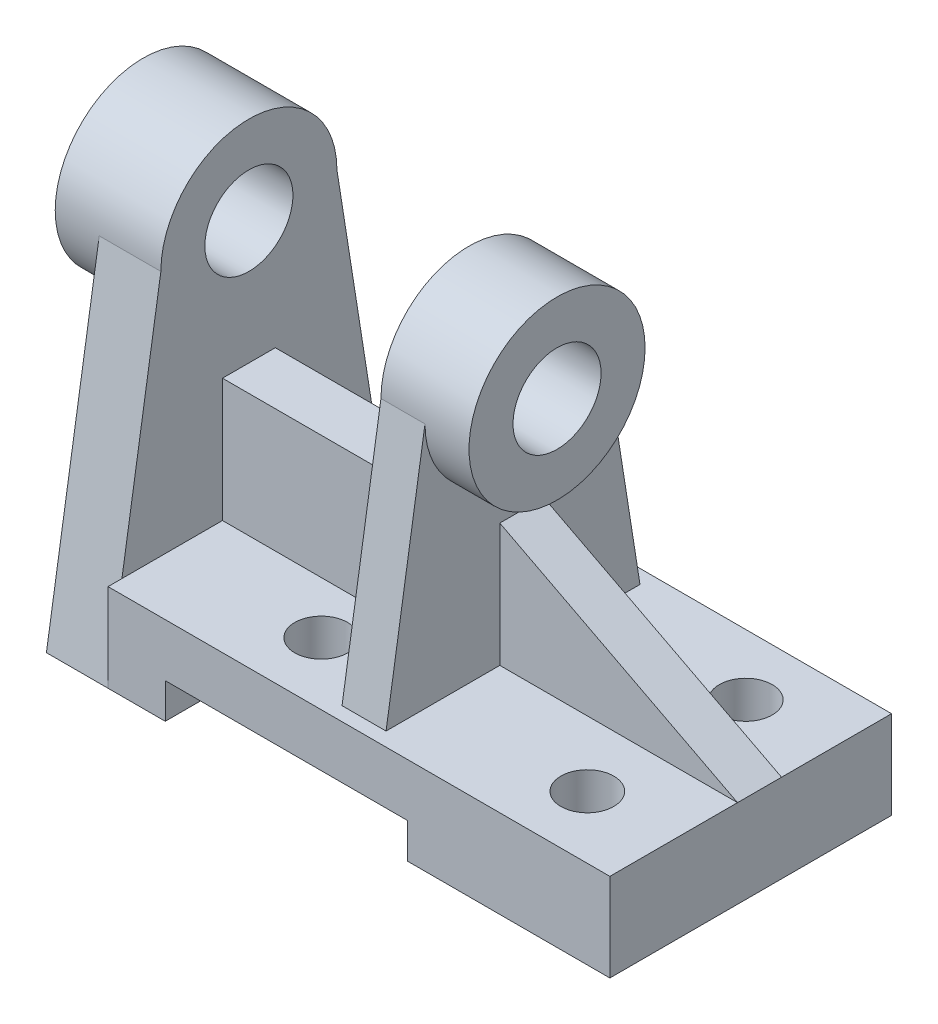
ISO-10303-21;
HEADER;
FILE_DESCRIPTION(('STEP AP214'),'2;1');
FILE_NAME('part.step','',(''),(''),'','','');
FILE_SCHEMA(('AUTOMOTIVE_DESIGN { 1 0 10303 214 1 1 1 1 }'));
ENDSEC;
DATA;
#1=APPLICATION_CONTEXT('core data for automotive mechanical design processes');
#2=APPLICATION_PROTOCOL_DEFINITION('international standard','automotive_design',2000,#1);
#3=PRODUCT_CONTEXT('',#1,'mechanical');
#4=PRODUCT('Part','Part','',(#3));
#5=PRODUCT_RELATED_PRODUCT_CATEGORY('part','',(#4));
#6=PRODUCT_DEFINITION_FORMATION('','',#4);
#7=PRODUCT_DEFINITION_CONTEXT('part definition',#1,'design');
#8=PRODUCT_DEFINITION('design','',#6,#7);
#9=PRODUCT_DEFINITION_SHAPE('','',#8);
#10=(LENGTH_UNIT() NAMED_UNIT(*) SI_UNIT(.MILLI.,.METRE.));
#11=(NAMED_UNIT(*) PLANE_ANGLE_UNIT() SI_UNIT($,.RADIAN.));
#12=(NAMED_UNIT(*) SI_UNIT($,.STERADIAN.) SOLID_ANGLE_UNIT());
#13=UNCERTAINTY_MEASURE_WITH_UNIT(LENGTH_MEASURE(1.E-05),#10,'distance_accuracy_value','');
#14=(GEOMETRIC_REPRESENTATION_CONTEXT(3) GLOBAL_UNCERTAINTY_ASSIGNED_CONTEXT((#13)) GLOBAL_UNIT_ASSIGNED_CONTEXT((#10,
#11,#12)) REPRESENTATION_CONTEXT('',''));
#15=CARTESIAN_POINT('',(0.,0.,0.));
#16=DIRECTION('',(0.,0.,1.));
#17=DIRECTION('',(1.,0.,0.));
#18=AXIS2_PLACEMENT_3D('',#15,#16,#17);
#19=CARTESIAN_POINT('',(-64.,10.,64.));
#20=DIRECTION('',(0.,-1.,0.));
#21=DIRECTION('',(1.,0.,0.));
#22=AXIS2_PLACEMENT_3D('',#19,#20,#21);
#23=PLANE('',#22);
#24=CARTESIAN_POINT('',(-15.7437869593848,10.,49.8283194926064));
#25=DIRECTION('',(0.,1.,0.));
#26=DIRECTION('',(-1.,0.,0.));
#27=AXIS2_PLACEMENT_3D('',#24,#25,#26);
#28=CIRCLE('',#27,6.);
#29=CARTESIAN_POINT('',(-21.7437869593848,10.,49.8283194926064));
#30=VERTEX_POINT('',#29);
#31=EDGE_CURVE('E223',#30,#30,#28,.T.);
#32=ORIENTED_EDGE('',*,*,#31,.F.);
#33=EDGE_LOOP('',(#32));
#34=FACE_BOUND('',#33,.T.);
#35=CARTESIAN_POINT('',(44.7041403429973,10.,49.8283194926064));
#36=DIRECTION('',(0.,1.,0.));
#37=DIRECTION('',(-1.,0.,0.));
#38=AXIS2_PLACEMENT_3D('',#35,#36,#37);
#39=CIRCLE('',#38,6.);
#40=CARTESIAN_POINT('',(38.7041403429973,10.,49.8283194926064));
#41=VERTEX_POINT('',#40);
#42=EDGE_CURVE('E495',#41,#41,#39,.T.);
#43=ORIENTED_EDGE('',*,*,#42,.F.);
#44=EDGE_LOOP('',(#43));
#45=FACE_BOUND('',#44,.T.);
#46=DIRECTION('',(0.,0.,-1.));
#47=VECTOR('',#46,1.);
#48=CARTESIAN_POINT('',(64.,10.,64.));
#49=LINE('',#48,#47);
#50=CARTESIAN_POINT('',(64.,10.,64.));
#51=VERTEX_POINT('',#50);
#52=CARTESIAN_POINT('',(64.,10.,35.));
#53=VERTEX_POINT('',#52);
#54=EDGE_CURVE('E385',#51,#53,#49,.T.);
#55=ORIENTED_EDGE('',*,*,#54,.T.);
#56=DIRECTION('',(-1.,0.,0.));
#57=VECTOR('',#56,1.);
#58=CARTESIAN_POINT('',(-64.,10.,35.));
#59=LINE('',#58,#57);
#60=CARTESIAN_POINT('',(10.,10.,35.));
#61=VERTEX_POINT('',#60);
#62=EDGE_CURVE('E236',#53,#61,#59,.T.);
#63=ORIENTED_EDGE('',*,*,#62,.T.);
#64=DIRECTION('',(0.,0.,-1.));
#65=VECTOR('',#64,1.);
#66=CARTESIAN_POINT('',(10.,10.,60.8421052631579));
#67=LINE('',#66,#65);
#68=CARTESIAN_POINT('',(10.,10.,60.8421052631579));
#69=VERTEX_POINT('',#68);
#70=EDGE_CURVE('E256',#69,#61,#67,.T.);
#71=ORIENTED_EDGE('',*,*,#70,.F.);
#72=DIRECTION('',(-1.,0.,0.));
#73=VECTOR('',#72,1.);
#74=CARTESIAN_POINT('',(10.,10.,60.8421052631579));
#75=LINE('',#74,#73);
#76=CARTESIAN_POINT('',(0.,10.,60.8421052631579));
#77=VERTEX_POINT('',#76);
#78=EDGE_CURVE('E271',#69,#77,#75,.T.);
#79=ORIENTED_EDGE('',*,*,#78,.T.);
#80=DIRECTION('',(0.,0.,-1.));
#81=VECTOR('',#80,1.);
#82=CARTESIAN_POINT('',(0.,10.,60.8421052631579));
#83=LINE('',#82,#81);
#84=CARTESIAN_POINT('',(0.,10.,38.));
#85=VERTEX_POINT('',#84);
#86=EDGE_CURVE('E264',#77,#85,#83,.T.);
#87=ORIENTED_EDGE('',*,*,#86,.T.);
#88=DIRECTION('',(1.,0.,0.));
#89=VECTOR('',#88,1.);
#90=CARTESIAN_POINT('',(0.,10.,38.));
#91=LINE('',#90,#89);
#92=CARTESIAN_POINT('',(-50.,10.,38.));
#93=VERTEX_POINT('',#92);
#94=EDGE_CURVE('E278',#93,#85,#91,.T.);
#95=ORIENTED_EDGE('',*,*,#94,.F.);
#96=DIRECTION('',(0.,0.,-1.));
#97=VECTOR('',#96,1.);
#98=CARTESIAN_POINT('',(-50.,10.,0.));
#99=LINE('',#98,#97);
#100=CARTESIAN_POINT('',(-50.,10.,60.8421052631579));
#101=VERTEX_POINT('',#100);
#102=EDGE_CURVE('E344',#101,#93,#99,.T.);
#103=ORIENTED_EDGE('',*,*,#102,.F.);
#104=CARTESIAN_POINT('',(-50.,10.,64.));
#105=VERTEX_POINT('',#104);
#106=EDGE_CURVE('E336',#105,#101,#99,.T.);
#107=ORIENTED_EDGE('',*,*,#106,.F.);
#108=DIRECTION('',(-1.,0.,0.));
#109=VECTOR('',#108,1.);
#110=CARTESIAN_POINT('',(-64.,10.,64.));
#111=LINE('',#110,#109);
#112=EDGE_CURVE('E359',#51,#105,#111,.T.);
#113=ORIENTED_EDGE('',*,*,#112,.F.);
#114=EDGE_LOOP('',(#55,#63,#71,#79,#87,#95,#103,#107,#113));
#115=FACE_BOUND('',#114,.T.);
#116=ADVANCED_FACE('F39',(#34,#45,#115),#23,.F.);
#117=CARTESIAN_POINT('',(0.,0.,0.));
#118=DIRECTION('',(1.,0.,0.));
#119=DIRECTION('',(0.,0.,-1.));
#120=AXIS2_PLACEMENT_3D('',#117,#118,#119);
#121=PLANE('',#120);
#122=DIRECTION('',(0.,-1.,0.));
#123=VECTOR('',#122,1.);
#124=CARTESIAN_POINT('',(0.,38.,26.));
#125=LINE('',#124,#123);
#126=CARTESIAN_POINT('',(0.,38.,26.));
#127=VERTEX_POINT('',#126);
#128=CARTESIAN_POINT('',(0.,10.,26.));
#129=VERTEX_POINT('',#128);
#130=EDGE_CURVE('E294',#127,#129,#125,.T.);
#131=ORIENTED_EDGE('',*,*,#130,.F.);
#132=DIRECTION('',(0.,0.,-1.));
#133=VECTOR('',#132,1.);
#134=CARTESIAN_POINT('',(0.,38.,26.));
#135=LINE('',#134,#133);
#136=CARTESIAN_POINT('',(0.,38.,38.));
#137=VERTEX_POINT('',#136);
#138=EDGE_CURVE('E284',#137,#127,#135,.T.);
#139=ORIENTED_EDGE('',*,*,#138,.F.);
#140=DIRECTION('',(0.,-1.,0.));
#141=VECTOR('',#140,1.);
#142=CARTESIAN_POINT('',(0.,38.,38.));
#143=LINE('',#142,#141);
#144=EDGE_CURVE('E296',#137,#85,#143,.T.);
#145=ORIENTED_EDGE('',*,*,#144,.T.);
#146=ORIENTED_EDGE('',*,*,#86,.F.);
#147=DIRECTION('',(0.,-0.987762965329069,0.155962573473011));
#148=VECTOR('',#147,1.);
#149=CARTESIAN_POINT('',(0.,66.,52.));
#150=LINE('',#149,#148);
#151=CARTESIAN_POINT('',(0.,66.,52.));
#152=VERTEX_POINT('',#151);
#153=EDGE_CURVE('E249',#152,#77,#150,.T.);
#154=ORIENTED_EDGE('',*,*,#153,.F.);
#155=CARTESIAN_POINT('',(0.,66.,32.));
#156=DIRECTION('',(1.,0.,0.));
#157=DIRECTION('',(0.,0.,-1.));
#158=AXIS2_PLACEMENT_3D('',#155,#156,#157);
#159=CIRCLE('',#158,20.);
#160=CARTESIAN_POINT('',(0.,66.,12.));
#161=VERTEX_POINT('',#160);
#162=EDGE_CURVE('E242',#161,#152,#159,.T.);
#163=ORIENTED_EDGE('',*,*,#162,.F.);
#164=DIRECTION('',(0.,0.987762965329069,0.155962573473011));
#165=VECTOR('',#164,1.);
#166=CARTESIAN_POINT('',(0.,10.,3.15789473684211));
#167=LINE('',#166,#165);
#168=CARTESIAN_POINT('',(0.,10.,3.15789473684211));
#169=VERTEX_POINT('',#168);
#170=EDGE_CURVE('E259',#169,#161,#167,.T.);
#171=ORIENTED_EDGE('',*,*,#170,.F.);
#172=EDGE_CURVE('E261',#129,#169,#83,.T.);
#173=ORIENTED_EDGE('',*,*,#172,.F.);
#174=EDGE_LOOP('',(#131,#139,#145,#146,#154,#163,#171,#173));
#175=FACE_BOUND('',#174,.T.);
#176=CARTESIAN_POINT('',(0.,66.,32.));
#177=DIRECTION('',(1.,0.,0.));
#178=DIRECTION('',(0.,0.,-1.));
#179=AXIS2_PLACEMENT_3D('',#176,#177,#178);
#180=CIRCLE('',#179,10.);
#181=CARTESIAN_POINT('',(0.,66.,22.));
#182=VERTEX_POINT('',#181);
#183=EDGE_CURVE('E239',#182,#182,#180,.T.);
#184=ORIENTED_EDGE('',*,*,#183,.T.);
#185=EDGE_LOOP('',(#184));
#186=FACE_BOUND('',#185,.T.);
#187=ADVANCED_FACE('F411',(#175,#186),#121,.F.);
#188=CARTESIAN_POINT('',(44.7041403429973,10.,13.8283194926064));
#189=DIRECTION('',(0.,1.,0.));
#190=DIRECTION('',(-1.,0.,0.));
#191=AXIS2_PLACEMENT_3D('',#188,#189,#190);
#192=CIRCLE('',#191,6.);
#193=CARTESIAN_POINT('',(38.7041403429973,10.,13.8283194926064));
#194=VERTEX_POINT('',#193);
#195=EDGE_CURVE('E235',#194,#194,#192,.T.);
#196=ORIENTED_EDGE('',*,*,#195,.F.);
#197=EDGE_LOOP('',(#196));
#198=FACE_BOUND('',#197,.T.);
#199=CARTESIAN_POINT('',(-15.7437869593848,10.,13.8283194926064));
#200=DIRECTION('',(0.,1.,0.));
#201=DIRECTION('',(-1.,0.,0.));
#202=AXIS2_PLACEMENT_3D('',#199,#200,#201);
#203=CIRCLE('',#202,6.);
#204=CARTESIAN_POINT('',(-21.7437869593848,10.,13.8283194926064));
#205=VERTEX_POINT('',#204);
#206=EDGE_CURVE('E216',#205,#205,#203,.T.);
#207=ORIENTED_EDGE('',*,*,#206,.F.);
#208=EDGE_LOOP('',(#207));
#209=FACE_BOUND('',#208,.T.);
#210=ORIENTED_EDGE('',*,*,#172,.T.);
#211=DIRECTION('',(-1.,0.,0.));
#212=VECTOR('',#211,1.);
#213=CARTESIAN_POINT('',(10.,10.,3.15789473684211));
#214=LINE('',#213,#212);
#215=CARTESIAN_POINT('',(10.,10.,3.15789473684211));
#216=VERTEX_POINT('',#215);
#217=EDGE_CURVE('E269',#216,#169,#214,.T.);
#218=ORIENTED_EDGE('',*,*,#217,.F.);
#219=CARTESIAN_POINT('',(10.,10.,25.));
#220=VERTEX_POINT('',#219);
#221=EDGE_CURVE('E253',#220,#216,#67,.T.);
#222=ORIENTED_EDGE('',*,*,#221,.F.);
#223=DIRECTION('',(-1.,0.,0.));
#224=VECTOR('',#223,1.);
#225=CARTESIAN_POINT('',(-64.,10.,25.));
#226=LINE('',#225,#224);
#227=CARTESIAN_POINT('',(64.,10.,25.));
#228=VERTEX_POINT('',#227);
#229=EDGE_CURVE('E57',#228,#220,#226,.T.);
#230=ORIENTED_EDGE('',*,*,#229,.F.);
#231=CARTESIAN_POINT('',(64.,10.,0.));
#232=VERTEX_POINT('',#231);
#233=EDGE_CURVE('E382',#228,#232,#49,.T.);
#234=ORIENTED_EDGE('',*,*,#233,.T.);
#235=DIRECTION('',(-1.,0.,0.));
#236=VECTOR('',#235,1.);
#237=CARTESIAN_POINT('',(-64.,10.,0.));
#238=LINE('',#237,#236);
#239=CARTESIAN_POINT('',(-50.,10.,0.));
#240=VERTEX_POINT('',#239);
#241=EDGE_CURVE('E371',#232,#240,#238,.T.);
#242=ORIENTED_EDGE('',*,*,#241,.T.);
#243=DIRECTION('',(0.,0.,-1.));
#244=VECTOR('',#243,1.);
#245=CARTESIAN_POINT('',(-50.,10.,64.));
#246=LINE('',#245,#244);
#247=CARTESIAN_POINT('',(-50.,10.,3.15789473684211));
#248=VERTEX_POINT('',#247);
#249=EDGE_CURVE('E309',#248,#240,#246,.T.);
#250=ORIENTED_EDGE('',*,*,#249,.F.);
#251=CARTESIAN_POINT('',(-50.,10.,26.));
#252=VERTEX_POINT('',#251);
#253=EDGE_CURVE('E340',#252,#248,#99,.T.);
#254=ORIENTED_EDGE('',*,*,#253,.F.);
#255=DIRECTION('',(-1.,0.,0.));
#256=VECTOR('',#255,1.);
#257=CARTESIAN_POINT('',(-50.,10.,26.));
#258=LINE('',#257,#256);
#259=EDGE_CURVE('E285',#129,#252,#258,.T.);
#260=ORIENTED_EDGE('',*,*,#259,.F.);
#261=EDGE_LOOP('',(#210,#218,#222,#230,#234,#242,#250,#254,#260));
#262=FACE_BOUND('',#261,.T.);
#263=ADVANCED_FACE('F430',(#198,#209,#262),#23,.F.);
#264=CARTESIAN_POINT('',(-50.,66.,0.));
#265=DIRECTION('',(-1.,0.,0.));
#266=DIRECTION('',(0.,-1.,0.));
#267=AXIS2_PLACEMENT_3D('',#264,#265,#266);
#268=PLANE('',#267);
#269=CARTESIAN_POINT('',(-50.,66.,32.));
#270=DIRECTION('',(-1.,0.,0.));
#271=DIRECTION('',(0.,0.,1.));
#272=AXIS2_PLACEMENT_3D('',#269,#270,#271);
#273=CIRCLE('',#272,10.);
#274=CARTESIAN_POINT('',(-50.,66.,42.));
#275=VERTEX_POINT('',#274);
#276=EDGE_CURVE('E325',#275,#275,#273,.T.);
#277=ORIENTED_EDGE('',*,*,#276,.T.);
#278=EDGE_LOOP('',(#277));
#279=FACE_BOUND('',#278,.T.);
#280=DIRECTION('',(0.,-1.,0.));
#281=VECTOR('',#280,1.);
#282=CARTESIAN_POINT('',(-50.,38.,38.));
#283=LINE('',#282,#281);
#284=CARTESIAN_POINT('',(-50.,38.,38.));
#285=VERTEX_POINT('',#284);
#286=EDGE_CURVE('E297',#285,#93,#283,.T.);
#287=ORIENTED_EDGE('',*,*,#286,.F.);
#288=DIRECTION('',(0.,0.,1.));
#289=VECTOR('',#288,1.);
#290=CARTESIAN_POINT('',(-50.,38.,38.));
#291=LINE('',#290,#289);
#292=CARTESIAN_POINT('',(-50.,38.,26.));
#293=VERTEX_POINT('',#292);
#294=EDGE_CURVE('E63',#293,#285,#291,.T.);
#295=ORIENTED_EDGE('',*,*,#294,.F.);
#296=DIRECTION('',(0.,-1.,0.));
#297=VECTOR('',#296,1.);
#298=CARTESIAN_POINT('',(-50.,38.,26.));
#299=LINE('',#298,#297);
#300=EDGE_CURVE('E288',#293,#252,#299,.T.);
#301=ORIENTED_EDGE('',*,*,#300,.T.);
#302=ORIENTED_EDGE('',*,*,#253,.T.);
#303=DIRECTION('',(0.,-0.987762965329069,-0.155962573473011));
#304=VECTOR('',#303,1.);
#305=CARTESIAN_POINT('',(-50.,-0.243243243243243,1.54054054054054));
#306=LINE('',#305,#304);
#307=CARTESIAN_POINT('',(-50.,66.,12.));
#308=VERTEX_POINT('',#307);
#309=EDGE_CURVE('E302',#308,#248,#306,.T.);
#310=ORIENTED_EDGE('',*,*,#309,.F.);
#311=CARTESIAN_POINT('',(-50.,66.,32.));
#312=DIRECTION('',(-1.,0.,0.));
#313=DIRECTION('',(0.,0.,1.));
#314=AXIS2_PLACEMENT_3D('',#311,#312,#313);
#315=CIRCLE('',#314,20.);
#316=CARTESIAN_POINT('',(-50.,66.,52.));
#317=VERTEX_POINT('',#316);
#318=EDGE_CURVE('E328',#317,#308,#315,.T.);
#319=ORIENTED_EDGE('',*,*,#318,.F.);
#320=DIRECTION('',(0.,0.987762965329069,-0.155962573473011));
#321=VECTOR('',#320,1.);
#322=CARTESIAN_POINT('',(-50.,9.61621621621621,60.9027027027027));
#323=LINE('',#322,#321);
#324=EDGE_CURVE('E319',#101,#317,#323,.T.);
#325=ORIENTED_EDGE('',*,*,#324,.F.);
#326=ORIENTED_EDGE('',*,*,#102,.T.);
#327=EDGE_LOOP('',(#287,#295,#301,#302,#310,#319,#325,#326));
#328=FACE_BOUND('',#327,.T.);
#329=ADVANCED_FACE('F446',(#279,#328),#268,.F.);
#330=CARTESIAN_POINT('',(0.,0.,64.));
#331=DIRECTION('',(0.,0.,1.));
#332=DIRECTION('',(1.,0.,0.));
#333=AXIS2_PLACEMENT_3D('',#330,#331,#332);
#334=PLANE('',#333);
#335=ORIENTED_EDGE('',*,*,#112,.T.);
#336=DIRECTION('',(0.,1.,0.));
#337=VECTOR('',#336,1.);
#338=CARTESIAN_POINT('',(-50.,0.,64.));
#339=LINE('',#338,#337);
#340=CARTESIAN_POINT('',(-50.,-9.99999999999999,64.));
#341=VERTEX_POINT('',#340);
#342=EDGE_CURVE('E313',#341,#105,#339,.T.);
#343=ORIENTED_EDGE('',*,*,#342,.F.);
#344=DIRECTION('',(1.,0.,0.));
#345=VECTOR('',#344,1.);
#346=CARTESIAN_POINT('',(-64.,-9.99999999999999,64.));
#347=LINE('',#346,#345);
#348=CARTESIAN_POINT('',(-37.,-9.99999999999999,64.));
#349=VERTEX_POINT('',#348);
#350=EDGE_CURVE('E368',#341,#349,#347,.T.);
#351=ORIENTED_EDGE('',*,*,#350,.T.);
#352=DIRECTION('',(0.,-1.,0.));
#353=VECTOR('',#352,1.);
#354=CARTESIAN_POINT('',(-37.,-9.99999999999999,64.));
#355=LINE('',#354,#353);
#356=CARTESIAN_POINT('',(-37.,-1.99999999999999,64.));
#357=VERTEX_POINT('',#356);
#358=EDGE_CURVE('E342',#357,#349,#355,.T.);
#359=ORIENTED_EDGE('',*,*,#358,.F.);
#360=DIRECTION('',(-1.,0.,0.));
#361=VECTOR('',#360,1.);
#362=CARTESIAN_POINT('',(-37.,-1.99999999999999,64.));
#363=LINE('',#362,#361);
#364=CARTESIAN_POINT('',(18.,-1.99999999999999,64.));
#365=VERTEX_POINT('',#364);
#366=EDGE_CURVE('E345',#365,#357,#363,.T.);
#367=ORIENTED_EDGE('',*,*,#366,.F.);
#368=DIRECTION('',(0.,1.,0.));
#369=VECTOR('',#368,1.);
#370=CARTESIAN_POINT('',(18.,-1.99999999999999,64.));
#371=LINE('',#370,#369);
#372=CARTESIAN_POINT('',(18.,-9.99999999999999,64.));
#373=VERTEX_POINT('',#372);
#374=EDGE_CURVE('E338',#373,#365,#371,.T.);
#375=ORIENTED_EDGE('',*,*,#374,.F.);
#376=CARTESIAN_POINT('',(64.,-9.99999999999999,64.));
#377=VERTEX_POINT('',#376);
#378=EDGE_CURVE('E364',#373,#377,#347,.T.);
#379=ORIENTED_EDGE('',*,*,#378,.T.);
#380=DIRECTION('',(0.,1.,0.));
#381=VECTOR('',#380,1.);
#382=CARTESIAN_POINT('',(64.,10.,64.));
#383=LINE('',#382,#381);
#384=EDGE_CURVE('E357',#377,#51,#383,.T.);
#385=ORIENTED_EDGE('',*,*,#384,.T.);
#386=EDGE_LOOP('',(#335,#343,#351,#359,#367,#375,#379,#385));
#387=FACE_BOUND('',#386,.T.);
#388=ADVANCED_FACE('F485',(#387),#334,.T.);
#389=CARTESIAN_POINT('',(0.,0.,0.));
#390=DIRECTION('',(0.,0.,1.));
#391=DIRECTION('',(1.,0.,0.));
#392=AXIS2_PLACEMENT_3D('',#389,#390,#391);
#393=PLANE('',#392);
#394=DIRECTION('',(0.,-1.,0.));
#395=VECTOR('',#394,1.);
#396=CARTESIAN_POINT('',(-50.,0.,0.));
#397=LINE('',#396,#395);
#398=CARTESIAN_POINT('',(-50.,-9.99999999999999,0.));
#399=VERTEX_POINT('',#398);
#400=EDGE_CURVE('E310',#240,#399,#397,.T.);
#401=ORIENTED_EDGE('',*,*,#400,.F.);
#402=ORIENTED_EDGE('',*,*,#241,.F.);
#403=DIRECTION('',(0.,1.,0.));
#404=VECTOR('',#403,1.);
#405=CARTESIAN_POINT('',(64.,10.,0.));
#406=LINE('',#405,#404);
#407=CARTESIAN_POINT('',(64.,-9.99999999999999,0.));
#408=VERTEX_POINT('',#407);
#409=EDGE_CURVE('E358',#408,#232,#406,.T.);
#410=ORIENTED_EDGE('',*,*,#409,.F.);
#411=DIRECTION('',(1.,0.,0.));
#412=VECTOR('',#411,1.);
#413=CARTESIAN_POINT('',(-64.,-9.99999999999999,0.));
#414=LINE('',#413,#412);
#415=CARTESIAN_POINT('',(18.,-9.99999999999999,0.));
#416=VERTEX_POINT('',#415);
#417=EDGE_CURVE('E372',#416,#408,#414,.T.);
#418=ORIENTED_EDGE('',*,*,#417,.F.);
#419=DIRECTION('',(0.,-1.,0.));
#420=VECTOR('',#419,1.);
#421=CARTESIAN_POINT('',(18.,0.,0.));
#422=LINE('',#421,#420);
#423=CARTESIAN_POINT('',(18.,-1.99999999999999,0.));
#424=VERTEX_POINT('',#423);
#425=EDGE_CURVE('E393',#424,#416,#422,.T.);
#426=ORIENTED_EDGE('',*,*,#425,.F.);
#427=DIRECTION('',(1.,0.,0.));
#428=VECTOR('',#427,1.);
#429=CARTESIAN_POINT('',(0.,-1.99999999999999,0.));
#430=LINE('',#429,#428);
#431=CARTESIAN_POINT('',(-37.,-1.99999999999999,0.));
#432=VERTEX_POINT('',#431);
#433=EDGE_CURVE('E390',#432,#424,#430,.T.);
#434=ORIENTED_EDGE('',*,*,#433,.F.);
#435=DIRECTION('',(0.,1.,0.));
#436=VECTOR('',#435,1.);
#437=CARTESIAN_POINT('',(-37.,0.,0.));
#438=LINE('',#437,#436);
#439=CARTESIAN_POINT('',(-37.,-9.99999999999999,0.));
#440=VERTEX_POINT('',#439);
#441=EDGE_CURVE('E383',#440,#432,#438,.T.);
#442=ORIENTED_EDGE('',*,*,#441,.F.);
#443=EDGE_CURVE('E380',#399,#440,#414,.T.);
#444=ORIENTED_EDGE('',*,*,#443,.F.);
#445=EDGE_LOOP('',(#401,#402,#410,#418,#426,#434,#442,#444));
#446=FACE_BOUND('',#445,.T.);
#447=ADVANCED_FACE('F431',(#446),#393,.F.);
#448=CARTESIAN_POINT('',(-64.,10.,64.));
#449=DIRECTION('',(1.,0.,0.));
#450=DIRECTION('',(0.,0.,-1.));
#451=AXIS2_PLACEMENT_3D('',#448,#449,#450);
#452=PLANE('',#451);
#453=DIRECTION('',(0.,0.987762965329069,-0.155962573473011));
#454=VECTOR('',#453,1.);
#455=CARTESIAN_POINT('',(-64.,9.61621621621621,60.9027027027027));
#456=LINE('',#455,#454);
#457=CARTESIAN_POINT('',(-64.,-9.99999999999999,64.));
#458=VERTEX_POINT('',#457);
#459=CARTESIAN_POINT('',(-64.,66.,52.));
#460=VERTEX_POINT('',#459);
#461=EDGE_CURVE('E303',#458,#460,#456,.T.);
#462=ORIENTED_EDGE('',*,*,#461,.T.);
#463=CARTESIAN_POINT('',(-64.,66.,32.));
#464=DIRECTION('',(1.,0.,0.));
#465=DIRECTION('',(0.,0.,-1.));
#466=AXIS2_PLACEMENT_3D('',#463,#464,#465);
#467=CIRCLE('',#466,20.);
#468=CARTESIAN_POINT('',(-64.,66.,12.));
#469=VERTEX_POINT('',#468);
#470=EDGE_CURVE('E334',#469,#460,#467,.F.);
#471=ORIENTED_EDGE('',*,*,#470,.F.);
#472=DIRECTION('',(0.,-0.987762965329069,-0.155962573473011));
#473=VECTOR('',#472,1.);
#474=CARTESIAN_POINT('',(-64.,-0.243243243243243,1.54054054054054));
#475=LINE('',#474,#473);
#476=CARTESIAN_POINT('',(-64.,-9.99999999999999,0.));
#477=VERTEX_POINT('',#476);
#478=EDGE_CURVE('E311',#469,#477,#475,.T.);
#479=ORIENTED_EDGE('',*,*,#478,.T.);
#480=DIRECTION('',(0.,0.,-1.));
#481=VECTOR('',#480,1.);
#482=CARTESIAN_POINT('',(-64.,-9.99999999999999,64.));
#483=LINE('',#482,#481);
#484=EDGE_CURVE('E378',#458,#477,#483,.T.);
#485=ORIENTED_EDGE('',*,*,#484,.F.);
#486=EDGE_LOOP('',(#462,#471,#479,#485));
#487=FACE_BOUND('',#486,.T.);
#488=ADVANCED_FACE('F566',(#487),#452,.F.);
#489=CARTESIAN_POINT('',(-64.,-9.99999999999999,64.));
#490=DIRECTION('',(0.,1.,0.));
#491=DIRECTION('',(0.,0.,1.));
#492=AXIS2_PLACEMENT_3D('',#489,#490,#491);
#493=PLANE('',#492);
#494=CARTESIAN_POINT('',(44.7041403429973,-9.99999999999999,13.8283194926064));
#495=DIRECTION('',(0.,1.,0.));
#496=DIRECTION('',(-1.,0.,0.));
#497=AXIS2_PLACEMENT_3D('',#494,#495,#496);
#498=CIRCLE('',#497,6.);
#499=CARTESIAN_POINT('',(38.7041403429973,-9.99999999999999,13.8283194926064));
#500=VERTEX_POINT('',#499);
#501=EDGE_CURVE('E226',#500,#500,#498,.T.);
#502=ORIENTED_EDGE('',*,*,#501,.T.);
#503=EDGE_LOOP('',(#502));
#504=FACE_BOUND('',#503,.T.);
#505=CARTESIAN_POINT('',(44.7041403429973,-9.99999999999999,49.8283194926064));
#506=DIRECTION('',(0.,1.,0.));
#507=DIRECTION('',(-1.,0.,0.));
#508=AXIS2_PLACEMENT_3D('',#505,#506,#507);
#509=CIRCLE('',#508,6.);
#510=CARTESIAN_POINT('',(38.7041403429973,-9.99999999999999,49.8283194926064));
#511=VERTEX_POINT('',#510);
#512=EDGE_CURVE('E490',#511,#511,#509,.T.);
#513=ORIENTED_EDGE('',*,*,#512,.T.);
#514=EDGE_LOOP('',(#513));
#515=FACE_BOUND('',#514,.T.);
#516=DIRECTION('',(0.,0.,-1.));
#517=VECTOR('',#516,1.);
#518=CARTESIAN_POINT('',(18.,-9.99999999999999,64.));
#519=LINE('',#518,#517);
#520=EDGE_CURVE('E352',#373,#416,#519,.T.);
#521=ORIENTED_EDGE('',*,*,#520,.T.);
#522=ORIENTED_EDGE('',*,*,#417,.T.);
#523=DIRECTION('',(0.,0.,-1.));
#524=VECTOR('',#523,1.);
#525=CARTESIAN_POINT('',(64.,-9.99999999999999,64.));
#526=LINE('',#525,#524);
#527=EDGE_CURVE('E370',#377,#408,#526,.T.);
#528=ORIENTED_EDGE('',*,*,#527,.F.);
#529=ORIENTED_EDGE('',*,*,#378,.F.);
#530=EDGE_LOOP('',(#521,#522,#528,#529));
#531=FACE_BOUND('',#530,.T.);
#532=ADVANCED_FACE('F569',(#504,#515,#531),#493,.F.);
#533=ORIENTED_EDGE('',*,*,#484,.T.);
#534=EDGE_CURVE('E363',#477,#399,#414,.T.);
#535=ORIENTED_EDGE('',*,*,#534,.T.);
#536=ORIENTED_EDGE('',*,*,#443,.T.);
#537=DIRECTION('',(0.,0.,-1.));
#538=VECTOR('',#537,1.);
#539=CARTESIAN_POINT('',(-37.,-9.99999999999999,64.));
#540=LINE('',#539,#538);
#541=EDGE_CURVE('E346',#349,#440,#540,.T.);
#542=ORIENTED_EDGE('',*,*,#541,.F.);
#543=ORIENTED_EDGE('',*,*,#350,.F.);
#544=EDGE_CURVE('E362',#458,#341,#347,.T.);
#545=ORIENTED_EDGE('',*,*,#544,.F.);
#546=EDGE_LOOP('',(#533,#535,#536,#542,#543,#545));
#547=FACE_BOUND('',#546,.T.);
#548=ADVANCED_FACE('F577',(#547),#493,.F.);
#549=CARTESIAN_POINT('',(64.,10.,64.));
#550=DIRECTION('',(-1.,0.,0.));
#551=DIRECTION('',(0.,0.,1.));
#552=AXIS2_PLACEMENT_3D('',#549,#550,#551);
#553=PLANE('',#552);
#554=ORIENTED_EDGE('',*,*,#527,.T.);
#555=ORIENTED_EDGE('',*,*,#409,.T.);
#556=ORIENTED_EDGE('',*,*,#233,.F.);
#557=DIRECTION('',(0.,0.,1.));
#558=VECTOR('',#557,1.);
#559=CARTESIAN_POINT('',(64.,10.,64.));
#560=LINE('',#559,#558);
#561=EDGE_CURVE('E206',#53,#228,#560,.F.);
#562=ORIENTED_EDGE('',*,*,#561,.F.);
#563=ORIENTED_EDGE('',*,*,#54,.F.);
#564=ORIENTED_EDGE('',*,*,#384,.F.);
#565=EDGE_LOOP('',(#554,#555,#556,#562,#563,#564));
#566=FACE_BOUND('',#565,.T.);
#567=ADVANCED_FACE('F41',(#566),#553,.F.);
#568=CARTESIAN_POINT('',(18.,-1.99999999999999,64.));
#569=DIRECTION('',(-1.,0.,0.));
#570=DIRECTION('',(0.,0.,1.));
#571=AXIS2_PLACEMENT_3D('',#568,#569,#570);
#572=PLANE('',#571);
#573=DIRECTION('',(0.,0.,-1.));
#574=VECTOR('',#573,1.);
#575=CARTESIAN_POINT('',(18.,-1.99999999999999,64.));
#576=LINE('',#575,#574);
#577=EDGE_CURVE('E355',#365,#424,#576,.T.);
#578=ORIENTED_EDGE('',*,*,#577,.T.);
#579=ORIENTED_EDGE('',*,*,#425,.T.);
#580=ORIENTED_EDGE('',*,*,#520,.F.);
#581=ORIENTED_EDGE('',*,*,#374,.T.);
#582=EDGE_LOOP('',(#578,#579,#580,#581));
#583=FACE_BOUND('',#582,.T.);
#584=ADVANCED_FACE('F589',(#583),#572,.T.);
#585=CARTESIAN_POINT('',(-37.,-1.99999999999999,64.));
#586=DIRECTION('',(0.,-1.,0.));
#587=DIRECTION('',(0.,0.,-1.));
#588=AXIS2_PLACEMENT_3D('',#585,#586,#587);
#589=PLANE('',#588);
#590=CARTESIAN_POINT('',(-15.7437869593848,-1.99999999999999,49.8283194926064));
#591=DIRECTION('',(0.,-1.,0.));
#592=DIRECTION('',(0.,0.,-1.));
#593=AXIS2_PLACEMENT_3D('',#590,#591,#592);
#594=CIRCLE('',#593,6.);
#595=CARTESIAN_POINT('',(-15.7437869593848,-1.99999999999999,43.8283194926064));
#596=VERTEX_POINT('',#595);
#597=EDGE_CURVE('E43',#596,#596,#594,.T.);
#598=ORIENTED_EDGE('',*,*,#597,.F.);
#599=EDGE_LOOP('',(#598));
#600=FACE_BOUND('',#599,.T.);
#601=CARTESIAN_POINT('',(-15.7437869593848,-1.99999999999999,13.8283194926064));
#602=DIRECTION('',(0.,-1.,0.));
#603=DIRECTION('',(0.,0.,-1.));
#604=AXIS2_PLACEMENT_3D('',#601,#602,#603);
#605=CIRCLE('',#604,6.);
#606=CARTESIAN_POINT('',(-15.7437869593848,-1.99999999999999,7.82831949260638));
#607=VERTEX_POINT('',#606);
#608=EDGE_CURVE('E218',#607,#607,#605,.T.);
#609=ORIENTED_EDGE('',*,*,#608,.F.);
#610=EDGE_LOOP('',(#609));
#611=FACE_BOUND('',#610,.T.);
#612=DIRECTION('',(0.,0.,-1.));
#613=VECTOR('',#612,1.);
#614=CARTESIAN_POINT('',(-37.,-1.99999999999999,64.));
#615=LINE('',#614,#613);
#616=EDGE_CURVE('E347',#357,#432,#615,.T.);
#617=ORIENTED_EDGE('',*,*,#616,.T.);
#618=ORIENTED_EDGE('',*,*,#433,.T.);
#619=ORIENTED_EDGE('',*,*,#577,.F.);
#620=ORIENTED_EDGE('',*,*,#366,.T.);
#621=EDGE_LOOP('',(#617,#618,#619,#620));
#622=FACE_BOUND('',#621,.T.);
#623=ADVANCED_FACE('F594',(#600,#611,#622),#589,.T.);
#624=CARTESIAN_POINT('',(-37.,-9.99999999999999,64.));
#625=DIRECTION('',(1.,0.,0.));
#626=DIRECTION('',(0.,0.,-1.));
#627=AXIS2_PLACEMENT_3D('',#624,#625,#626);
#628=PLANE('',#627);
#629=ORIENTED_EDGE('',*,*,#541,.T.);
#630=ORIENTED_EDGE('',*,*,#441,.T.);
#631=ORIENTED_EDGE('',*,*,#616,.F.);
#632=ORIENTED_EDGE('',*,*,#358,.T.);
#633=EDGE_LOOP('',(#629,#630,#631,#632));
#634=FACE_BOUND('',#633,.T.);
#635=ADVANCED_FACE('F605',(#634),#628,.T.);
#636=CARTESIAN_POINT('',(-74.,66.,32.));
#637=DIRECTION('',(-1.,0.,0.));
#638=DIRECTION('',(0.,0.,1.));
#639=AXIS2_PLACEMENT_3D('',#636,#637,#638);
#640=PLANE('',#639);
#641=CARTESIAN_POINT('',(-74.,66.,32.));
#642=DIRECTION('',(-1.,0.,0.));
#643=DIRECTION('',(0.,0.,1.));
#644=AXIS2_PLACEMENT_3D('',#641,#642,#643);
#645=CIRCLE('',#644,10.);
#646=CARTESIAN_POINT('',(-74.,66.,42.));
#647=VERTEX_POINT('',#646);
#648=EDGE_CURVE('E329',#647,#647,#645,.T.);
#649=ORIENTED_EDGE('',*,*,#648,.F.);
#650=EDGE_LOOP('',(#649));
#651=FACE_BOUND('',#650,.T.);
#652=CARTESIAN_POINT('',(-74.,66.,32.));
#653=DIRECTION('',(-1.,0.,0.));
#654=DIRECTION('',(0.,0.,1.));
#655=AXIS2_PLACEMENT_3D('',#652,#653,#654);
#656=CIRCLE('',#655,20.);
#657=CARTESIAN_POINT('',(-74.,66.,52.));
#658=VERTEX_POINT('',#657);
#659=EDGE_CURVE('E335',#658,#658,#656,.T.);
#660=ORIENTED_EDGE('',*,*,#659,.T.);
#661=EDGE_LOOP('',(#660));
#662=FACE_BOUND('',#661,.T.);
#663=ADVANCED_FACE('F610',(#651,#662),#640,.T.);
#664=CARTESIAN_POINT('',(-74.,66.,32.));
#665=DIRECTION('',(1.,0.,0.));
#666=DIRECTION('',(0.,0.,-1.));
#667=AXIS2_PLACEMENT_3D('',#664,#665,#666);
#668=CYLINDRICAL_SURFACE('',#667,20.);
#669=ORIENTED_EDGE('',*,*,#470,.T.);
#670=DIRECTION('',(1.,0.,0.));
#671=VECTOR('',#670,1.);
#672=CARTESIAN_POINT('',(-74.,66.,52.));
#673=LINE('',#672,#671);
#674=EDGE_CURVE('E396',#317,#460,#673,.F.);
#675=ORIENTED_EDGE('',*,*,#674,.F.);
#676=ORIENTED_EDGE('',*,*,#318,.T.);
#677=DIRECTION('',(1.,0.,0.));
#678=VECTOR('',#677,1.);
#679=CARTESIAN_POINT('',(-74.,66.,12.));
#680=LINE('',#679,#678);
#681=EDGE_CURVE('E394',#469,#308,#680,.T.);
#682=ORIENTED_EDGE('',*,*,#681,.F.);
#683=EDGE_LOOP('',(#669,#675,#676,#682));
#684=FACE_BOUND('',#683,.T.);
#685=ORIENTED_EDGE('',*,*,#659,.F.);
#686=EDGE_LOOP('',(#685));
#687=FACE_BOUND('',#686,.T.);
#688=ADVANCED_FACE('F618',(#684,#687),#668,.T.);
#689=CARTESIAN_POINT('',(-74.,66.,32.));
#690=DIRECTION('',(1.,0.,0.));
#691=DIRECTION('',(0.,0.,-1.));
#692=AXIS2_PLACEMENT_3D('',#689,#690,#691);
#693=CYLINDRICAL_SURFACE('',#692,10.);
#694=ORIENTED_EDGE('',*,*,#276,.F.);
#695=EDGE_LOOP('',(#694));
#696=FACE_BOUND('',#695,.T.);
#697=ORIENTED_EDGE('',*,*,#648,.T.);
#698=EDGE_LOOP('',(#697));
#699=FACE_BOUND('',#698,.T.);
#700=ADVANCED_FACE('F622',(#696,#699),#693,.F.);
#701=CARTESIAN_POINT('',(-50.,0.,0.));
#702=DIRECTION('',(-1.,0.,0.));
#703=DIRECTION('',(0.,0.,1.));
#704=AXIS2_PLACEMENT_3D('',#701,#702,#703);
#705=PLANE('',#704);
#706=ORIENTED_EDGE('',*,*,#106,.T.);
#707=EDGE_CURVE('E314',#341,#101,#323,.T.);
#708=ORIENTED_EDGE('',*,*,#707,.F.);
#709=ORIENTED_EDGE('',*,*,#342,.T.);
#710=EDGE_LOOP('',(#706,#708,#709));
#711=FACE_BOUND('',#710,.T.);
#712=ADVANCED_FACE('F634',(#711),#705,.T.);
#713=CARTESIAN_POINT('',(-50.,9.61621621621621,60.9027027027027));
#714=DIRECTION('',(0.,0.155962573473011,0.987762965329069));
#715=DIRECTION('',(0.,-0.987762965329069,0.155962573473011));
#716=AXIS2_PLACEMENT_3D('',#713,#714,#715);
#717=PLANE('',#716);
#718=ORIENTED_EDGE('',*,*,#461,.F.);
#719=ORIENTED_EDGE('',*,*,#544,.T.);
#720=ORIENTED_EDGE('',*,*,#707,.T.);
#721=ORIENTED_EDGE('',*,*,#324,.T.);
#722=ORIENTED_EDGE('',*,*,#674,.T.);
#723=EDGE_LOOP('',(#718,#719,#720,#721,#722));
#724=FACE_BOUND('',#723,.T.);
#725=ADVANCED_FACE('F736',(#724),#717,.T.);
#726=CARTESIAN_POINT('',(-50.,0.,0.));
#727=DIRECTION('',(-1.,0.,0.));
#728=DIRECTION('',(0.,0.,1.));
#729=AXIS2_PLACEMENT_3D('',#726,#727,#728);
#730=PLANE('',#729);
#731=ORIENTED_EDGE('',*,*,#249,.T.);
#732=ORIENTED_EDGE('',*,*,#400,.T.);
#733=EDGE_CURVE('E308',#248,#399,#306,.T.);
#734=ORIENTED_EDGE('',*,*,#733,.F.);
#735=EDGE_LOOP('',(#731,#732,#734));
#736=FACE_BOUND('',#735,.T.);
#737=ADVANCED_FACE('F437',(#736),#730,.T.);
#738=CARTESIAN_POINT('',(-50.,-0.243243243243243,1.54054054054054));
#739=DIRECTION('',(0.,0.155962573473011,-0.987762965329069));
#740=DIRECTION('',(0.,0.987762965329069,0.155962573473011));
#741=AXIS2_PLACEMENT_3D('',#738,#739,#740);
#742=PLANE('',#741);
#743=ORIENTED_EDGE('',*,*,#478,.F.);
#744=ORIENTED_EDGE('',*,*,#681,.T.);
#745=ORIENTED_EDGE('',*,*,#309,.T.);
#746=ORIENTED_EDGE('',*,*,#733,.T.);
#747=ORIENTED_EDGE('',*,*,#534,.F.);
#748=EDGE_LOOP('',(#743,#744,#745,#746,#747));
#749=FACE_BOUND('',#748,.T.);
#750=ADVANCED_FACE('F445',(#749),#742,.T.);
#751=CARTESIAN_POINT('',(0.,38.,38.));
#752=DIRECTION('',(0.,0.,-1.));
#753=DIRECTION('',(-1.,0.,0.));
#754=AXIS2_PLACEMENT_3D('',#751,#752,#753);
#755=PLANE('',#754);
#756=ORIENTED_EDGE('',*,*,#94,.T.);
#757=ORIENTED_EDGE('',*,*,#144,.F.);
#758=DIRECTION('',(1.,0.,0.));
#759=VECTOR('',#758,1.);
#760=CARTESIAN_POINT('',(0.,38.,38.));
#761=LINE('',#760,#759);
#762=EDGE_CURVE('E283',#285,#137,#761,.T.);
#763=ORIENTED_EDGE('',*,*,#762,.F.);
#764=ORIENTED_EDGE('',*,*,#286,.T.);
#765=EDGE_LOOP('',(#756,#757,#763,#764));
#766=FACE_BOUND('',#765,.T.);
#767=ADVANCED_FACE('F759',(#766),#755,.F.);
#768=CARTESIAN_POINT('',(-50.,38.,26.));
#769=DIRECTION('',(0.,0.,1.));
#770=DIRECTION('',(1.,0.,0.));
#771=AXIS2_PLACEMENT_3D('',#768,#769,#770);
#772=PLANE('',#771);
#773=ORIENTED_EDGE('',*,*,#259,.T.);
#774=ORIENTED_EDGE('',*,*,#300,.F.);
#775=DIRECTION('',(-1.,0.,0.));
#776=VECTOR('',#775,1.);
#777=CARTESIAN_POINT('',(-50.,38.,26.));
#778=LINE('',#777,#776);
#779=EDGE_CURVE('E286',#127,#293,#778,.T.);
#780=ORIENTED_EDGE('',*,*,#779,.F.);
#781=ORIENTED_EDGE('',*,*,#130,.T.);
#782=EDGE_LOOP('',(#773,#774,#780,#781));
#783=FACE_BOUND('',#782,.T.);
#784=ADVANCED_FACE('F451',(#783),#772,.F.);
#785=CARTESIAN_POINT('',(0.,38.,0.));
#786=DIRECTION('',(0.,-1.,0.));
#787=DIRECTION('',(1.,0.,0.));
#788=AXIS2_PLACEMENT_3D('',#785,#786,#787);
#789=PLANE('',#788);
#790=ORIENTED_EDGE('',*,*,#138,.T.);
#791=ORIENTED_EDGE('',*,*,#779,.T.);
#792=ORIENTED_EDGE('',*,*,#294,.T.);
#793=ORIENTED_EDGE('',*,*,#762,.T.);
#794=EDGE_LOOP('',(#790,#791,#792,#793));
#795=FACE_BOUND('',#794,.T.);
#796=ADVANCED_FACE('F462',(#795),#789,.F.);
#797=CARTESIAN_POINT('',(10.,66.,52.));
#798=DIRECTION('',(0.,-0.155962573473011,-0.987762965329069));
#799=DIRECTION('',(0.,0.987762965329069,-0.155962573473011));
#800=AXIS2_PLACEMENT_3D('',#797,#798,#799);
#801=PLANE('',#800);
#802=ORIENTED_EDGE('',*,*,#153,.T.);
#803=ORIENTED_EDGE('',*,*,#78,.F.);
#804=DIRECTION('',(0.,-0.987762965329069,0.155962573473011));
#805=VECTOR('',#804,1.);
#806=CARTESIAN_POINT('',(10.,66.,52.));
#807=LINE('',#806,#805);
#808=CARTESIAN_POINT('',(10.,66.,52.));
#809=VERTEX_POINT('',#808);
#810=EDGE_CURVE('E254',#809,#69,#807,.T.);
#811=ORIENTED_EDGE('',*,*,#810,.F.);
#812=DIRECTION('',(-1.,0.,0.));
#813=VECTOR('',#812,1.);
#814=CARTESIAN_POINT('',(10.,66.,52.));
#815=LINE('',#814,#813);
#816=EDGE_CURVE('E279',#809,#152,#815,.T.);
#817=ORIENTED_EDGE('',*,*,#816,.T.);
#818=EDGE_LOOP('',(#802,#803,#811,#817));
#819=FACE_BOUND('',#818,.T.);
#820=ADVANCED_FACE('F409',(#819),#801,.F.);
#821=CARTESIAN_POINT('',(10.,10.,3.15789473684211));
#822=DIRECTION('',(0.,-0.155962573473011,0.987762965329069));
#823=DIRECTION('',(0.,-0.987762965329069,-0.155962573473011));
#824=AXIS2_PLACEMENT_3D('',#821,#822,#823);
#825=PLANE('',#824);
#826=ORIENTED_EDGE('',*,*,#170,.T.);
#827=DIRECTION('',(-1.,0.,0.));
#828=VECTOR('',#827,1.);
#829=CARTESIAN_POINT('',(10.,66.,12.));
#830=LINE('',#829,#828);
#831=CARTESIAN_POINT('',(10.,66.,12.));
#832=VERTEX_POINT('',#831);
#833=EDGE_CURVE('E263',#832,#161,#830,.T.);
#834=ORIENTED_EDGE('',*,*,#833,.F.);
#835=DIRECTION('',(0.,0.987762965329069,0.155962573473011));
#836=VECTOR('',#835,1.);
#837=CARTESIAN_POINT('',(10.,10.,3.15789473684211));
#838=LINE('',#837,#836);
#839=EDGE_CURVE('E258',#216,#832,#838,.T.);
#840=ORIENTED_EDGE('',*,*,#839,.F.);
#841=ORIENTED_EDGE('',*,*,#217,.T.);
#842=EDGE_LOOP('',(#826,#834,#840,#841));
#843=FACE_BOUND('',#842,.T.);
#844=ADVANCED_FACE('F452',(#843),#825,.F.);
#845=CARTESIAN_POINT('',(10.,0.,0.));
#846=DIRECTION('',(1.,0.,0.));
#847=DIRECTION('',(0.,0.,-1.));
#848=AXIS2_PLACEMENT_3D('',#845,#846,#847);
#849=PLANE('',#848);
#850=DIRECTION('',(0.,-1.,0.));
#851=VECTOR('',#850,1.);
#852=CARTESIAN_POINT('',(10.,0.,35.));
#853=LINE('',#852,#851);
#854=CARTESIAN_POINT('',(10.,38.,35.));
#855=VERTEX_POINT('',#854);
#856=EDGE_CURVE('E11',#855,#61,#853,.T.);
#857=ORIENTED_EDGE('',*,*,#856,.F.);
#858=DIRECTION('',(0.,0.,-1.));
#859=VECTOR('',#858,1.);
#860=CARTESIAN_POINT('',(10.,38.,0.));
#861=LINE('',#860,#859);
#862=CARTESIAN_POINT('',(10.,38.,25.));
#863=VERTEX_POINT('',#862);
#864=EDGE_CURVE('E48',#863,#855,#861,.F.);
#865=ORIENTED_EDGE('',*,*,#864,.F.);
#866=DIRECTION('',(0.,-1.,0.));
#867=VECTOR('',#866,1.);
#868=CARTESIAN_POINT('',(10.,0.,25.));
#869=LINE('',#868,#867);
#870=EDGE_CURVE('E193',#863,#220,#869,.T.);
#871=ORIENTED_EDGE('',*,*,#870,.T.);
#872=ORIENTED_EDGE('',*,*,#221,.T.);
#873=ORIENTED_EDGE('',*,*,#839,.T.);
#874=CARTESIAN_POINT('',(10.,66.,32.));
#875=DIRECTION('',(1.,0.,0.));
#876=DIRECTION('',(0.,0.,-1.));
#877=AXIS2_PLACEMENT_3D('',#874,#875,#876);
#878=CIRCLE('',#877,20.);
#879=EDGE_CURVE('E201',#832,#809,#878,.F.);
#880=ORIENTED_EDGE('',*,*,#879,.T.);
#881=ORIENTED_EDGE('',*,*,#810,.T.);
#882=ORIENTED_EDGE('',*,*,#70,.T.);
#883=EDGE_LOOP('',(#857,#865,#871,#872,#873,#880,#881,#882));
#884=FACE_BOUND('',#883,.T.);
#885=ADVANCED_FACE('F211',(#884),#849,.T.);
#886=CARTESIAN_POINT('',(20.,66.,32.));
#887=DIRECTION('',(-1.,0.,0.));
#888=DIRECTION('',(0.,0.,1.));
#889=AXIS2_PLACEMENT_3D('',#886,#887,#888);
#890=CYLINDRICAL_SURFACE('',#889,20.);
#891=CARTESIAN_POINT('',(20.,66.,32.));
#892=DIRECTION('',(1.,0.,0.));
#893=DIRECTION('',(0.,0.,-1.));
#894=AXIS2_PLACEMENT_3D('',#891,#892,#893);
#895=CIRCLE('',#894,20.);
#896=CARTESIAN_POINT('',(20.,66.,12.));
#897=VERTEX_POINT('',#896);
#898=EDGE_CURVE('E250',#897,#897,#895,.T.);
#899=ORIENTED_EDGE('',*,*,#898,.F.);
#900=EDGE_LOOP('',(#899));
#901=FACE_BOUND('',#900,.T.);
#902=ORIENTED_EDGE('',*,*,#162,.T.);
#903=ORIENTED_EDGE('',*,*,#816,.F.);
#904=ORIENTED_EDGE('',*,*,#879,.F.);
#905=ORIENTED_EDGE('',*,*,#833,.T.);
#906=EDGE_LOOP('',(#902,#903,#904,#905));
#907=FACE_BOUND('',#906,.T.);
#908=ADVANCED_FACE('F410',(#901,#907),#890,.T.);
#909=CARTESIAN_POINT('',(20.,66.,32.));
#910=DIRECTION('',(-1.,0.,0.));
#911=DIRECTION('',(0.,0.,1.));
#912=AXIS2_PLACEMENT_3D('',#909,#910,#911);
#913=CYLINDRICAL_SURFACE('',#912,10.);
#914=ORIENTED_EDGE('',*,*,#183,.F.);
#915=EDGE_LOOP('',(#914));
#916=FACE_BOUND('',#915,.T.);
#917=CARTESIAN_POINT('',(20.,66.,32.));
#918=DIRECTION('',(1.,0.,0.));
#919=DIRECTION('',(0.,0.,-1.));
#920=AXIS2_PLACEMENT_3D('',#917,#918,#919);
#921=CIRCLE('',#920,10.);
#922=CARTESIAN_POINT('',(20.,66.,22.));
#923=VERTEX_POINT('',#922);
#924=EDGE_CURVE('E241',#923,#923,#921,.T.);
#925=ORIENTED_EDGE('',*,*,#924,.T.);
#926=EDGE_LOOP('',(#925));
#927=FACE_BOUND('',#926,.T.);
#928=ADVANCED_FACE('F524',(#916,#927),#913,.F.);
#929=CARTESIAN_POINT('',(20.,66.,32.));
#930=DIRECTION('',(1.,0.,0.));
#931=DIRECTION('',(0.,0.,-1.));
#932=AXIS2_PLACEMENT_3D('',#929,#930,#931);
#933=PLANE('',#932);
#934=ORIENTED_EDGE('',*,*,#898,.T.);
#935=EDGE_LOOP('',(#934));
#936=FACE_BOUND('',#935,.T.);
#937=ORIENTED_EDGE('',*,*,#924,.F.);
#938=EDGE_LOOP('',(#937));
#939=FACE_BOUND('',#938,.T.);
#940=ADVANCED_FACE('F517',(#936,#939),#933,.T.);
#941=CARTESIAN_POINT('',(-4.99999999999997,38.,35.));
#942=DIRECTION('',(0.,0.,1.));
#943=DIRECTION('',(1.,0.,0.));
#944=AXIS2_PLACEMENT_3D('',#941,#942,#943);
#945=PLANE('',#944);
#946=ORIENTED_EDGE('',*,*,#62,.F.);
#947=DIRECTION('',(0.88775453144893,-0.460317164455,0.));
#948=VECTOR('',#947,1.);
#949=CARTESIAN_POINT('',(10.,38.,35.));
#950=LINE('',#949,#948);
#951=EDGE_CURVE('E209',#855,#53,#950,.T.);
#952=ORIENTED_EDGE('',*,*,#951,.F.);
#953=ORIENTED_EDGE('',*,*,#856,.T.);
#954=EDGE_LOOP('',(#946,#952,#953));
#955=FACE_BOUND('',#954,.T.);
#956=ADVANCED_FACE('F419',(#955),#945,.T.);
#957=CARTESIAN_POINT('',(-4.99999999999997,38.,25.));
#958=DIRECTION('',(0.,0.,1.));
#959=DIRECTION('',(1.,0.,0.));
#960=AXIS2_PLACEMENT_3D('',#957,#958,#959);
#961=PLANE('',#960);
#962=DIRECTION('',(0.88775453144893,-0.460317164455,0.));
#963=VECTOR('',#962,1.);
#964=CARTESIAN_POINT('',(10.,38.,25.));
#965=LINE('',#964,#963);
#966=EDGE_CURVE('E200',#863,#228,#965,.T.);
#967=ORIENTED_EDGE('',*,*,#966,.T.);
#968=ORIENTED_EDGE('',*,*,#229,.T.);
#969=ORIENTED_EDGE('',*,*,#870,.F.);
#970=EDGE_LOOP('',(#967,#968,#969));
#971=FACE_BOUND('',#970,.T.);
#972=ADVANCED_FACE('F198',(#971),#961,.F.);
#973=CARTESIAN_POINT('',(10.,38.,30.));
#974=DIRECTION('',(-0.460317164455,-0.88775453144893,0.));
#975=DIRECTION('',(0.88775453144893,-0.460317164455,0.));
#976=AXIS2_PLACEMENT_3D('',#973,#974,#975);
#977=PLANE('',#976);
#978=ORIENTED_EDGE('',*,*,#951,.T.);
#979=ORIENTED_EDGE('',*,*,#561,.T.);
#980=ORIENTED_EDGE('',*,*,#966,.F.);
#981=ORIENTED_EDGE('',*,*,#864,.T.);
#982=EDGE_LOOP('',(#978,#979,#980,#981));
#983=FACE_BOUND('',#982,.T.);
#984=ADVANCED_FACE('F204',(#983),#977,.F.);
#985=CARTESIAN_POINT('',(-15.7437869593848,-9.99999999999999,13.8283194926064));
#986=DIRECTION('',(0.,1.,0.));
#987=DIRECTION('',(-1.,0.,0.));
#988=AXIS2_PLACEMENT_3D('',#985,#986,#987);
#989=CYLINDRICAL_SURFACE('',#988,6.);
#990=ORIENTED_EDGE('',*,*,#608,.T.);
#991=EDGE_LOOP('',(#990));
#992=FACE_BOUND('',#991,.T.);
#993=ORIENTED_EDGE('',*,*,#206,.T.);
#994=EDGE_LOOP('',(#993));
#995=FACE_BOUND('',#994,.T.);
#996=ADVANCED_FACE('F515',(#992,#995),#989,.F.);
#997=CARTESIAN_POINT('',(-15.7437869593848,-9.99999999999999,49.8283194926064));
#998=DIRECTION('',(0.,1.,0.));
#999=DIRECTION('',(-1.,0.,0.));
#1000=AXIS2_PLACEMENT_3D('',#997,#998,#999);
#1001=CYLINDRICAL_SURFACE('',#1000,6.);
#1002=ORIENTED_EDGE('',*,*,#597,.T.);
#1003=EDGE_LOOP('',(#1002));
#1004=FACE_BOUND('',#1003,.T.);
#1005=ORIENTED_EDGE('',*,*,#31,.T.);
#1006=EDGE_LOOP('',(#1005));
#1007=FACE_BOUND('',#1006,.T.);
#1008=ADVANCED_FACE('F503',(#1004,#1007),#1001,.F.);
#1009=CARTESIAN_POINT('',(44.7041403429973,-9.99999999999999,49.8283194926064));
#1010=DIRECTION('',(0.,1.,0.));
#1011=DIRECTION('',(-1.,0.,0.));
#1012=AXIS2_PLACEMENT_3D('',#1009,#1010,#1011);
#1013=CYLINDRICAL_SURFACE('',#1012,6.);
#1014=ORIENTED_EDGE('',*,*,#512,.F.);
#1015=EDGE_LOOP('',(#1014));
#1016=FACE_BOUND('',#1015,.T.);
#1017=ORIENTED_EDGE('',*,*,#42,.T.);
#1018=EDGE_LOOP('',(#1017));
#1019=FACE_BOUND('',#1018,.T.);
#1020=ADVANCED_FACE('F499',(#1016,#1019),#1013,.F.);
#1021=CARTESIAN_POINT('',(44.7041403429973,-9.99999999999999,13.8283194926064));
#1022=DIRECTION('',(0.,1.,0.));
#1023=DIRECTION('',(-1.,0.,0.));
#1024=AXIS2_PLACEMENT_3D('',#1021,#1022,#1023);
#1025=CYLINDRICAL_SURFACE('',#1024,6.);
#1026=ORIENTED_EDGE('',*,*,#501,.F.);
#1027=EDGE_LOOP('',(#1026));
#1028=FACE_BOUND('',#1027,.T.);
#1029=ORIENTED_EDGE('',*,*,#195,.T.);
#1030=EDGE_LOOP('',(#1029));
#1031=FACE_BOUND('',#1030,.T.);
#1032=ADVANCED_FACE('F505',(#1028,#1031),#1025,.F.);
#1033=CLOSED_SHELL('',(#116,#187,#263,#329,#388,#447,#488,#532,#548,#567,#584,#623,#635,#663,
#688,#700,#712,#725,#737,#750,#767,#784,#796,#820,#844,#885,#908,#928,#940,#956,#972,#984,#996,
#1008,#1020,#1032));
#1034=MANIFOLD_SOLID_BREP('B2',#1033);
#1035=ADVANCED_BREP_SHAPE_REPRESENTATION('',(#18,#1034),#14);
#1036=SHAPE_DEFINITION_REPRESENTATION(#9,#1035);
ENDSEC;
END-ISO-10303-21;
